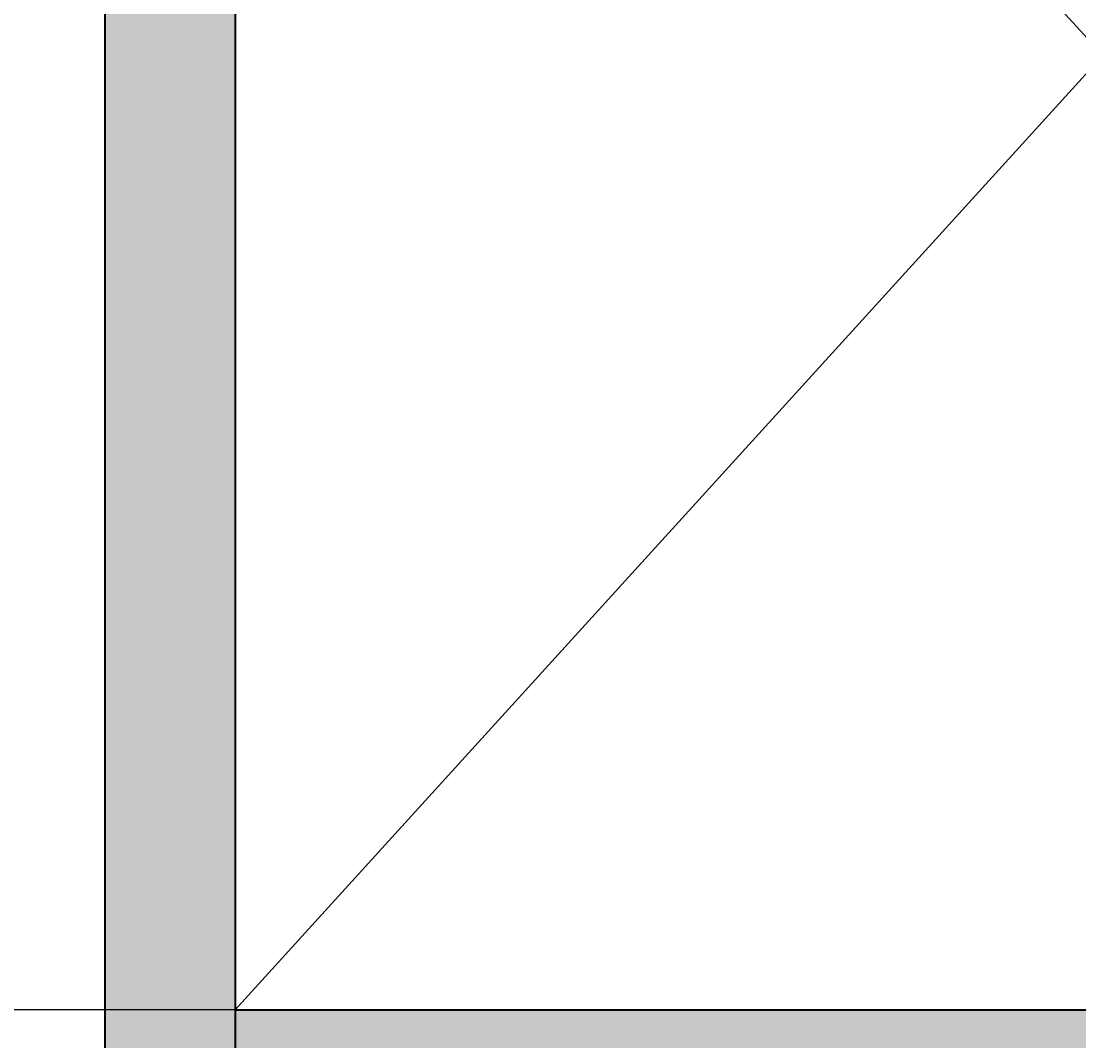
# Model space of a CAD drawing. Units: inches. Extents: x 1998 to 2588, y 1139 to 1977.
# Tile 32 of 134: x 2220 to 2257, y 1522 to 1557. Entities that reach past the tile are written whole.
import ezdxf

# ---------------------------------------------------------------- set-up
doc = ezdxf.new("R2010")
doc.units = ezdxf.units.IN
for name, color, linetype, lineweight in [('A-ANNO-DIMS', 2, 'Continuous', 18), ('A-FLOR-OPEN', 8, 'Continuous', 18), ('A-WALL-PATT', 252, 'Continuous', 13), ('WALL', 200, 'Continuous', 35)]:
    doc.layers.add(name, color=color, linetype=linetype, lineweight=lineweight)
doc.styles.get("Standard").update_dxf_attribs({"font": 'arial.ttf'})
doc.dimstyles.get("Standard").update_dxf_attribs({"dimtxt": 0.18, "dimasz": 0.18, "dimexe": 0.18, "dimexo": 0.0625, "dimgap": 0.09, "dimtad": 0, "dimtih": 1, "dimtoh": 1, "dimdec": 4, "dimzin": 0, "dimdsep": 46, "dimtxsty": 'Standard', "dimcen": 0.09, "dimadec": 0, "dimazin": 0, "dimtfac": 1, "dimtdec": 4, "dimtofl": 0, "dimtmove": 0, "dimatfit": 3, "dimfxl": 1, "dimtolj": 1, "dimtzin": 0, "dimarcsym": 0})

# ---------------------------------------------------------------- blocks, each defined once
blk = doc.blocks.new('*D34')
at = {"layer": 'A-ANNO-DIMS', "color": 0, "lineweight": -2, "transparency": 16777216}
for p, q in [((2407.91, 1594.732), (1997.843, 1594.732)), ((1998.023, 1594.552), (1998.023, 1558.913)), ((1998.023, 1522.912), (1998.023, 1558.552)), ((2407.91, 1522.732), (1997.843, 1522.732))]:
    blk.add_line(p, q, dxfattribs=at)
at = {"layer": 'A-ANNO-DIMS', "color": 0, "transparency": 16777216}
for points in [[(1997.993, 1594.552), (1998.053, 1594.552), (1998.023, 1594.732)], [(1997.993, 1522.912), (1998.053, 1522.912), (1998.023, 1522.732)]]:
    blk.add_solid(points, dxfattribs=at)
at = {"layer": 'Defpoints', "color": 0, "transparency": 16777216}
for p in [(1998.023, 1594.732), (2407.973, 1594.732), (2407.973, 1522.732)]:
    blk.add_point(p, dxfattribs=at)
at = {"layer": 'A-ANNO-DIMS', "color": 0, "transparency": 16777216, "insert": (1998.023, 1558.732), "char_height": 0.18, "attachment_point": 5}
blk.add_mtext('\\A1;72', dxfattribs=at)
blk = doc.blocks.new('*D41')
at = {"layer": 'A-ANNO-DIMS', "color": 0, "lineweight": -2, "transparency": 16777216}
for p, q in [((2227.473, 1588.67), (2227.473, 1138.602)), ((2287.473, 1588.67), (2287.473, 1138.602)), ((2227.653, 1138.782), (2257.254, 1138.782)), ((2287.293, 1138.782), (2257.692, 1138.782))]:
    blk.add_line(p, q, dxfattribs=at)
at = {"layer": 'A-ANNO-DIMS', "color": 0, "transparency": 16777216}
for points in [[(2227.653, 1138.812), (2227.653, 1138.752), (2227.473, 1138.782)], [(2287.293, 1138.812), (2287.293, 1138.752), (2287.473, 1138.782)]]:
    blk.add_solid(points, dxfattribs=at)
at = {"layer": 'Defpoints', "color": 0, "transparency": 16777216}
for p in [(2227.473, 1588.732), (2287.473, 1588.732), (2287.473, 1138.782)]:
    blk.add_point(p, dxfattribs=at)
at = {"layer": 'A-ANNO-DIMS', "color": 0, "transparency": 16777216, "insert": (2257.473, 1138.782), "char_height": 0.18, "attachment_point": 5}
blk.add_mtext('\\A1;60', dxfattribs=at)

msp = doc.modelspace()

# ---------------------------------------------------------------- hatches: boundary and pattern name
at = {"layer": 'A-WALL-PATT'}
h = msp.add_hatch(color=256, dxfattribs=at)
h.dxf.hatch_style = 1
h.paths.add_polyline_path([(2222.9729, 1888.7324), (2099.4125, 1888.7324), (2099.4125, 1879.7324), (2222.9729, 1879.7324)])
h.paths.add_polyline_path([(2096.9729, 1868.3278), (2087.9729, 1868.3278), (2087.9729, 1775.637), (2096.9729, 1775.637)])
h.paths.add_polyline_path([(2227.4729, 1868.3278), (2222.9729, 1868.3278), (2222.9729, 1774.3318), (2227.4729, 1774.3318)])
h.paths.add_polyline_path([(2188.3019, 1759.7324), (2138.6074, 1759.7324), (2099.4125, 1759.7324), (2099.4125, 1755.2324), (2176.9729, 1755.2324), (2188.3019, 1755.2324)])
h.paths.add_polyline_path([(2087.9729, 1759.7324), (2059.4729, 1759.7324), (2059.4729, 1702.7324), (2087.9729, 1702.7324), (2087.9729, 1707.2324), (2063.9729, 1707.2324), (2063.9729, 1755.2324), (2087.9729, 1755.2324)])
h.paths.add_polyline_path([(2096.9729, 1755.2324), (2087.9729, 1755.2324), (2087.9729, 1707.2324), (2096.9729, 1707.2324)])
h.paths.add_polyline_path([(2187.0461, 1707.2324), (2105.9729, 1707.2324), (2096.9729, 1707.2324), (2087.9729, 1707.2324), (2087.9729, 1702.7324), (2105.9729, 1702.7324), (2114.9729, 1702.7324), (2187.0461, 1702.7324)])
h.paths.add_polyline_path([(2181.4729, 1719.2028), (2176.9729, 1719.2028), (2176.9729, 1707.2324), (2181.4729, 1707.2324)])
h.paths.add_polyline_path([(2216.0332, 1588.7324), (2114.9729, 1588.7324), (2105.9729, 1588.7324), (2105.9729, 1584.2324), (2216.0332, 1584.2324)])
h.paths.add_polyline_path([(2077.691, 1588.7324), (2061.4729, 1588.7324), (2061.4729, 1584.2324), (2077.691, 1584.2324)])
h.paths.add_polyline_path([(2105.9729, 1588.7324), (2098.0956, 1588.7324), (2098.0956, 1584.2324), (2105.9729, 1584.2324)])
h.paths.add_polyline_path([(2114.9729, 1596.2642), (2110.1012, 1596.2642), (2105.9729, 1596.2642), (2105.9729, 1588.7324), (2114.9729, 1588.7324)])
h.paths.add_polyline_path([(2114.9729, 1584.2324), (2105.9729, 1584.2324), (2105.9729, 1580.249), (2110.1012, 1580.249), (2114.9729, 1580.249)])
h.paths.add_polyline_path([(2114.9729, 1547.7716), (2110.1012, 1547.7716, -0.0318759), (2105.9729, 1548.035), (2105.9729, 1470.2324), (2108.3775, 1470.2324), (2108.3775, 1465.7324), (2186.2943, 1465.7324), (2186.2943, 1470.2324), (2114.9729, 1470.2324)])
h.paths.add_polyline_path([(2227.4729, 1584.2324), (2222.9729, 1584.2324), (2222.9729, 1486.137), (2227.4729, 1486.137)])
h.paths.add_polyline_path([(2295.4138, 1593.2324), (2227.4729, 1593.2324), (2227.4729, 1588.7324), (2295.4138, 1588.7324), (2295.4138, 1591.8729)])
h.paths.add_polyline_path([(2345.9729, 1627.1165), (2341.4729, 1627.1165), (2341.4729, 1593.2324), (2337.2869, 1593.2324), (2337.2869, 1591.8729), (2337.2869, 1588.7324), (2345.9729, 1588.7324)])
h.paths.add_polyline_path([(2291.9729, 1588.7324), (2287.4729, 1588.7324), (2287.4729, 1522.7324), (2291.9729, 1522.7324)])
h.paths.add_polyline_path([(2291.9729, 1522.7324), (2287.4729, 1522.7324), (2227.4729, 1522.7324), (2227.4729, 1518.2324), (2291.9729, 1518.2324)])
h.paths.add_polyline_path([(2295.7347, 1519.5919), (2295.7347, 1522.7324), (2291.9729, 1522.7324), (2291.9729, 1518.2324), (2295.7347, 1518.2324)])
h.paths.add_polyline_path([(2345.9729, 1522.7324), (2337.6078, 1522.7324), (2337.6078, 1519.5919), (2337.6078, 1518.2324), (2341.4729, 1518.2324), (2341.4729, 1488.5616), (2345.9729, 1488.5616)])
h.paths.add_polyline_path([(2345.9729, 1468.1569), (2341.4729, 1468.1569), (2341.4729, 1374.2324), (2227.4729, 1374.2324), (2227.4729, 1369.7324), (2345.9729, 1369.7324)])
h.paths.add_polyline_path([(2345.9729, 1369.7324), (2341.4729, 1369.7324), (2341.4729, 1362.2324), (2345.9729, 1362.2324)])
h.paths.add_polyline_path([(2345.9729, 1317.7324), (2345.9729, 1322.2324), (2341.4729, 1322.2324), (2341.4729, 1285.137), (2345.9729, 1285.137)], flags=17)
h.paths.add_polyline_path([(2356.2096, 1322.2324), (2345.9729, 1322.2324), (2345.9729, 1317.7324), (2356.2096, 1317.7324), (2356.2096, 1319.3088)], flags=17)
h.paths.add_polyline_path([(2393.9729, 1322.2324), (2375.6999, 1322.2324), (2375.6999, 1319.3088, -0.0202458), (2375.636, 1317.7324), (2393.9729, 1317.7324)], flags=17)
h.paths.add_polyline_path([(2398.4729, 1322.2324), (2393.9729, 1322.2324), (2393.9729, 1317.7324), (2393.9729, 1237.7324), (2345.9729, 1237.7324), (2345.9729, 1264.7324), (2341.4729, 1264.7324), (2341.4729, 1228.7324), (2393.9729, 1228.7324), (2482.7412, 1228.7324), (2482.7412, 1237.7324), (2398.4729, 1237.7324), (2398.4729, 1297.1029)])
h.paths.add_polyline_path([(2398.4729, 1362.2324), (2393.9729, 1362.2324), (2393.9729, 1357.7324), (2398.4729, 1357.7324)])
h.paths.add_polyline_path([(2345.9729, 1329.7549), (2341.4729, 1329.7549), (2341.4729, 1322.2324), (2345.9729, 1322.2324)])

# ---------------------------------------------------------------- linework, layer by layer
at = {"layer": 'A-FLOR-OPEN'}
for p, q in [((2227.4729, 1522.7324), (2287.4729, 1588.7324)), ((2227.4729, 1588.7324), (2287.4729, 1522.7324))]:
    msp.add_line(p, q, dxfattribs=at)
at = {"layer": 'WALL'}
for p, q in [((2227.4729, 1588.7324), (2227.4729, 1486.137)), ((2227.4729, 1588.7324), (2227.4729, 1522.7324)), ((2222.9729, 1584.2324), (2222.9729, 1486.137)), ((2227.4729, 1522.7324), (2287.4729, 1522.7324)), ((2227.4729, 1522.7324), (2295.7347, 1522.7324))]:
    msp.add_line(p, q, dxfattribs=at)

# ---------------------------------------------------------------- dimensions: what is measured, and where the dimension line sits
at = {"layer": 'A-ANNO-DIMS'}
dim = msp.add_linear_dim(base=(1998.0229, 1594.7324), p1=(2407.9729, 1522.7324), p2=(2407.9729, 1594.7324), angle=90, dimstyle='Standard', override={"dimdec": 0, "dimlfac": 1, "dimrnd": 0, "dimzin": 0, "dimdsep": 46, "dimlunit": 2}, dxfattribs=at)
dim.commit()
dim.dimension.update_dxf_attribs({"geometry": '*D34', "text_midpoint": (1998.0229, 1558.7324)})
dim = msp.add_linear_dim(base=(2287.4729, 1138.7824), p1=(2227.4729, 1588.7324), p2=(2287.4729, 1588.7324), dimstyle='Standard', override={"dimdec": 0, "dimlfac": 1, "dimrnd": 0, "dimzin": 0, "dimdsep": 46, "dimlunit": 2}, dxfattribs=at)
dim.commit()
dim.dimension.update_dxf_attribs({"geometry": '*D41', "text_midpoint": (2257.4729, 1138.7824)})

doc.saveas('drawing.dxf')
